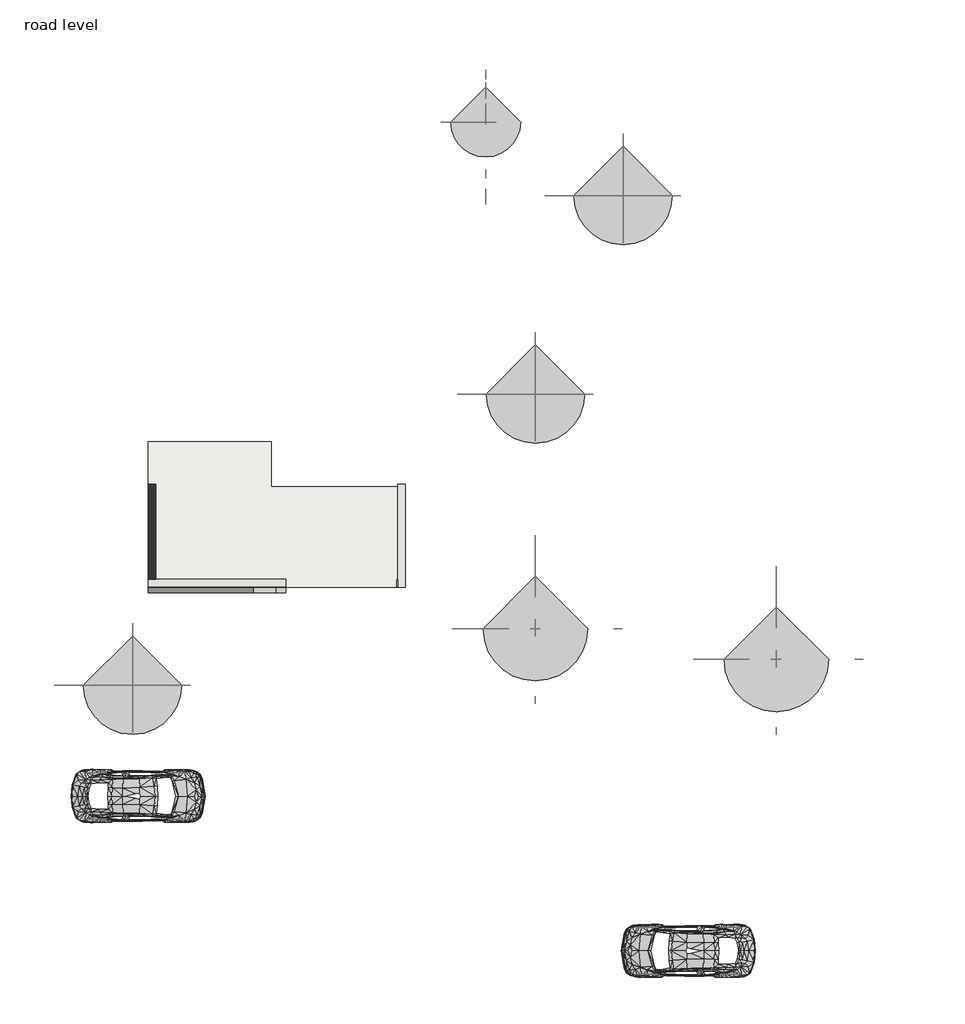
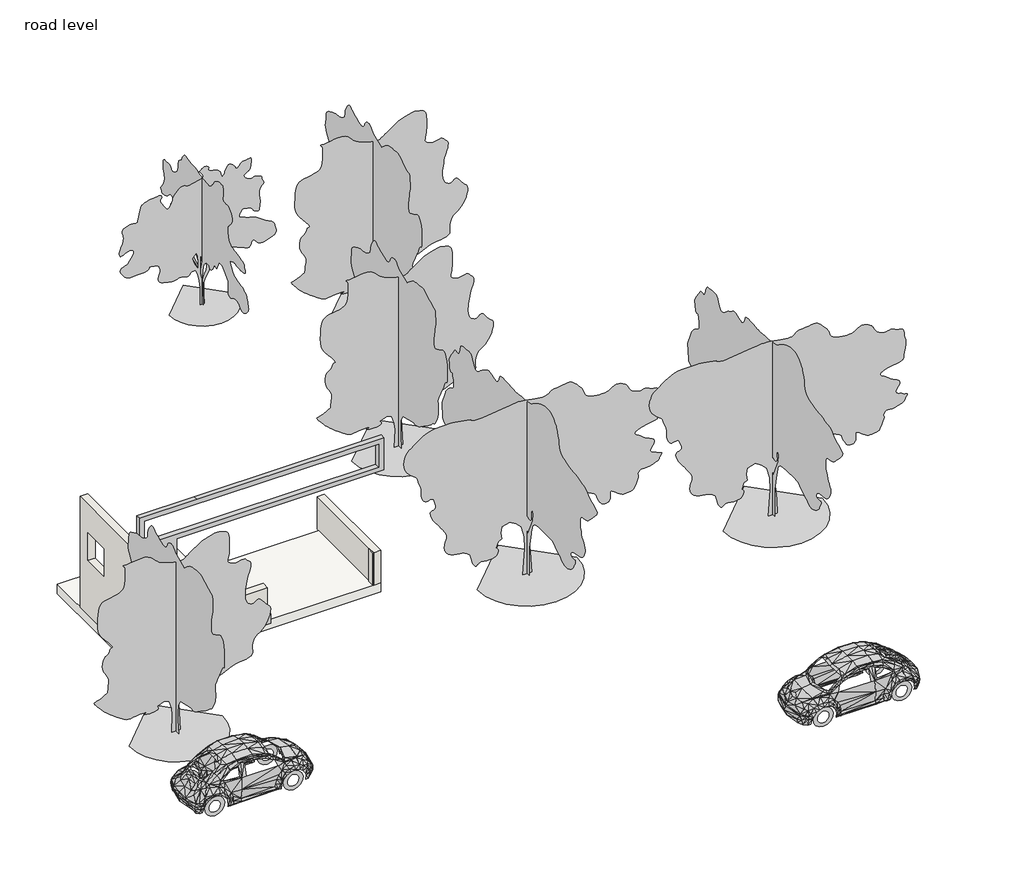
# One storey, incomplete: 6 geographic elements, 4 walls, 2 proxies, 1 furniture element, 1 slab.
"""IFC4 building model written with IfcOpenShell, lengths in millimetres."""

from ifc_helpers import new_model, si_unit, frame, origin, origin_with_axes, place, context, project, spatial, polyline, outline, extrude, faceted_brep, transform, mapped, element, save
from components import rpc_beetle_rpc_beetle_31f8b51e, casework_1_casework_1_0d475414, rpc_tree_deciduous_american_beech_20_b3c041c8, rpc_tree_deciduous_blue_berry_elder_15_a2d70376, rpc_tree_deciduous_common_apple_20_2cf08d23

model = new_model("IFC4")

# Units and contexts
model_context = context("Model", 3, world=origin())
ifc_project = project(units=[si_unit("LENGTHUNIT", "METRE", prefix="MILLI")], contexts=[model_context])

# Site, building, storey
site = spatial("IfcSite", under=ifc_project)
building = spatial("IfcBuilding", under=site)
storey = spatial("IfcBuildingStorey", under=building, Name="road level", Elevation=0.0)

# Proxies
placement = place(None, origin())
rpc_beetle_rpc_beetle_shape = rpc_beetle_rpc_beetle_31f8b51e(model_context)
element("IfcBuildingElementProxy", 1, Name="RPC Beetle : RPC Beetle", ObjectType="RPC Beetle : RPC Beetle", at=placement, inside=storey, context=model_context, shape_type="MappedRepresentation", body=[
    mapped(rpc_beetle_rpc_beetle_shape, transform((36221.8136801, -7466.6247213, -304.8), x_axis=(0.0, 1.0, 0.0), y_axis=(-1.0, 0.0, 0.0), z_axis=(0.0, 0.0, 1.0))),
])
element("IfcBuildingElementProxy", 2, Name="RPC Beetle : RPC Beetle", ObjectType="RPC Beetle : RPC Beetle", at=placement, inside=storey, context=model_context, shape_type="MappedRepresentation", body=[
    mapped(rpc_beetle_rpc_beetle_shape, transform((17489.3136801, -2887.1590687, -304.8), x_axis=(0.0, -1.0, 0.0), y_axis=(1.0, 0.0, 0.0), z_axis=(0.0, 0.0, 1.0))),
])

# Furniture
casework_1_casework_1_shape = casework_1_casework_1_0d475414(model_context)
element("IfcFurniture", 3, ObjectType="Casework 1 : Casework 1", at=placement, inside=storey, context=model_context, shape_type="MappedRepresentation", body=[
    mapped(casework_1_casework_1_shape, transform((0.0, 0.0, 0.0), x_axis=(1.0, 0.0, 0.0), y_axis=(0.0, 1.0, 0.0), z_axis=(0.0, 0.0, 1.0))),
])

# Geographic elements
rpc_tree_deciduous_american_beech_20_shape = rpc_tree_deciduous_american_beech_20_b3c041c8(model_context)
element("IfcGeographicElement", 4, ObjectType="RPC Tree - Deciduous : American Beech - 20'", at=placement, inside=storey, context=model_context, shape_type="MappedRepresentation", body=[
    mapped(rpc_tree_deciduous_american_beech_20_shape, transform((30470.0886189, 9000.0409313, -304.8), x_axis=(1.0, 0.0, 0.0), y_axis=(0.0, 1.0, 0.0), z_axis=(0.0, 0.0, 1.0))),
])
element("IfcGeographicElement", 5, ObjectType="RPC Tree - Deciduous : American Beech - 20'", at=placement, inside=storey, context=model_context, shape_type="MappedRepresentation", body=[
    mapped(rpc_tree_deciduous_american_beech_20_shape, transform((33060.8886189, 14867.4409313, -304.8), x_axis=(1.0, 0.0, 0.0), y_axis=(0.0, 1.0, 0.0), z_axis=(0.0, 0.0, 1.0))),
])
element("IfcGeographicElement", 6, ObjectType="RPC Tree - Deciduous : American Beech - 20'", at=placement, inside=storey, context=model_context, shape_type="MappedRepresentation", body=[
    mapped(rpc_tree_deciduous_american_beech_20_shape, transform((18556.1136801, 389.4409313, -304.8), x_axis=(1.0, 0.0, 0.0), y_axis=(0.0, 1.0, 0.0), z_axis=(0.0, 0.0, 1.0))),
])
rpc_tree_deciduous_blue_berry_elder_15_shape = rpc_tree_deciduous_blue_berry_elder_15_a2d70376(model_context)
element("IfcGeographicElement", 7, ObjectType="RPC Tree - Deciduous : Blue Berry Elder - 15'", at=placement, inside=storey, context=model_context, shape_type="MappedRepresentation", body=[
    mapped(rpc_tree_deciduous_blue_berry_elder_15_shape, transform((28995.5136801, 17044.3752787, 0.0), x_axis=(1.0, 0.0, 0.0), y_axis=(0.0, 1.0, 0.0), z_axis=(0.0, 0.0, 1.0))),
])
rpc_tree_deciduous_common_apple_20_shape = rpc_tree_deciduous_common_apple_20_2cf08d23(model_context)
element("IfcGeographicElement", 8, ObjectType="RPC Tree - Deciduous : Common Apple - 20'", at=placement, inside=storey, context=model_context, shape_type="MappedRepresentation", body=[
    mapped(rpc_tree_deciduous_common_apple_20_shape, transform((37593.4136801, 1151.4409313, -304.8), x_axis=(1.0, 0.0, 0.0), y_axis=(0.0, 1.0, 0.0), z_axis=(0.0, 0.0, 1.0))),
])
element("IfcGeographicElement", 9, ObjectType="RPC Tree - Deciduous : Common Apple - 20'", at=placement, inside=storey, context=model_context, shape_type="MappedRepresentation", body=[
    mapped(rpc_tree_deciduous_common_apple_20_shape, transform((30470.0886189, 2065.8409313, -304.8), x_axis=(1.0, 0.0, 0.0), y_axis=(0.0, 1.0, 0.0), z_axis=(0.0, 0.0, 1.0))),
])

# Slab
element("IfcSlab", 10, ObjectType="Generic - 12\"", at=placement, inside=storey, context=model_context, shape_type="SweptSolid", body=[
    extrude(outline(polyline([(19025.4925873, 7585.6570707), (22657.6925873, 7585.6570707), (22657.6925873, 6256.0880342), (26620.0925873, 6256.0880342), (26620.0925873, 3293.0570707), (19025.4925873, 3293.0570707), (19025.4925873, 7585.6570707)])), frame((0.0, 0.0, -304.8), z_axis=(0.0, 0.0, 1.0), x_axis=(1.0, 0.0, 0.0)), (0.0, 0.0, 1.0), 304.8),
])

# Walls
element("IfcWall", 11, at=placement, inside=storey, context=model_context, shape_type="SweptSolid", body=[
    extrude(outline(polyline([(26366.6136801, 3513.6409313), (26392.0136801, 3513.6409313), (26392.0136801, 3285.0409313), (26366.6136801, 3285.0409313), (26366.6136801, 3513.6409313)])), origin_with_axes(), (0.0, 0.0, 1.0), 1066.8),
])
element("IfcWall", 12, at=placement, inside=storey, context=model_context, shape_type="Brep", body=[
    faceted_brep([(19241.9136801, 3523.1659313, 0.0), (19241.9136801, 6333.0409313, 0.0), (19241.9136801, 6333.0409313, 3657.6), (19241.9136801, 4369.7752787, 3657.6), (19241.9136801, 3523.1659313, 3657.6), (19241.9136801, 5926.6409313, 2708.275), (19241.9136801, 5926.6409313, 1793.875), (19241.9136801, 5063.0409313, 1793.875), (19241.9136801, 5063.0409313, 2708.275), (19013.3136801, 3523.1659313, 0.0), (19013.3136801, 3523.1659313, 1066.8), (19013.3136801, 3523.1659313, 3657.6), (19013.3136801, 6333.0409313, 3657.6), (19013.3136801, 6333.0409313, 609.6), (19013.3136801, 6333.0409313, 0.0), (19013.3136801, 5926.6409313, 2708.275), (19013.3136801, 5063.0409313, 2708.275), (19013.3136801, 5063.0409313, 1793.875), (19013.3136801, 5926.6409313, 1793.875)], [[[0, 1, 2, 3, 4], [5, 6, 7, 8]], [[9, 10, 11, 12, 13, 14], [15, 16, 17, 18]], [[1, 0, 9, 14]], [[0, 4, 11, 10, 9]], [[2, 1, 14, 13, 12]], [[4, 3, 2, 12, 11]], [[6, 5, 15, 18]], [[7, 6, 18, 17]], [[8, 7, 17, 16]], [[5, 8, 16, 15]]]),
])
element("IfcWall", 13, at=placement, inside=storey, context=model_context, shape_type="Brep", body=[
    faceted_brep([(26392.0136801, 6333.0409313, 0.0), (26392.0136801, 3513.6409313, 0.0), (26392.0136801, 3285.0409313, 0.0), (26392.0136801, 3285.0409313, 1066.8), (26392.0136801, 3513.6409313, 1066.8), (26392.0136801, 6333.0409313, 1066.8), (26392.0136801, 6333.0409313, 609.6), (26620.6136801, 6333.0409313, 0.0), (26620.6136801, 6333.0409313, 609.6), (26620.6136801, 6333.0409313, 1066.8), (26620.6136801, 3285.0409313, 1066.8), (26620.6136801, 3285.0409313, 0.0)], [[[0, 1, 2, 3, 4, 5, 6]], [[7, 8, 9, 10, 11]], [[2, 1, 0, 7, 11]], [[5, 4, 3, 10, 9]], [[3, 2, 11, 10]], [[0, 6, 5, 9, 8, 7]]]),
])
element("IfcWall", 14, at=placement, inside=storey, context=model_context, shape_type="Brep", body=[
    faceted_brep([(23090.0136801, 3523.1659313, 0.0), (19241.9136801, 3523.1659313, 0.0), (19013.3136801, 3523.1659313, 0.0), (19013.3136801, 3523.1659313, 1066.8), (23090.0136801, 3523.1659313, 1066.8), (23090.0136801, 3294.5659313, 0.0), (23090.0136801, 3294.5659313, 1066.8), (19013.3136801, 3294.5659313, 1066.8), (19013.3136801, 3294.5659313, 0.0)], [[[0, 1, 2, 3, 4]], [[5, 6, 7, 8]], [[2, 1, 0, 5, 8]], [[4, 3, 7, 6]], [[0, 4, 6, 5]], [[3, 2, 8, 7]]]),
])

save(model, "model.ifc")

# Revit data of these elements
# Type "RPC Beetle : RPC Beetle"
#   built-in parameter 1005198 = "{2, 15},{39, RPC-16-0U6E-L4EG-ENH1-J3KF-SVEL-0TX4-C0},{1, 0},{1, 0},{2, 36},{1, 8},{5, Color},{1, 0},{1, 0},{3, 0.8},{3, 0.8},{3, 0.8},{1, 8},{7, BBoxMin},{1, 0},{1, 0},{1, 0},{1, 0},{1, 0},{1, 8},{7, BBoxMax},{1, 0},{1, 0},{1, 0},{1, 0},{1, 0},{2, 11},{9, RPCTypeId},{1, 0},{1, 0},{39, RPC-16-0U6E-L4EG-ENH1-J3KF-SVEL-0TX4-C0},{1, 6},{14, RPCPlantHeight},{1, 0},{1, 0},{7, 4.91667},{2, 11},{20, AdvancedUIDefinition},{1, 0},{1, 0},{0, },{2, 11},{10, AssetLibID},{1, 0},{1, 0},{36, 4D3F6E72-3F99-4203-98E9-AF80B3C7A7A4},{2, 11},{10, BaseSchema},{1, 0},{1, 0},{9, RPCSchema},{2, 11},{12, ExchangeGUID},{1, 0},{1, 0},{0, },{1, 2},{6, Hidden},{1, 0},{1, 0},{1, 0},{2, 11},{12, LocalizedUID},{1, 0},{1, 0},{0, },{1, 4},{11, RPCCategory},{1, 0},{1, 0},{1, 0},{2, 11},{8, RPCImage},{1, 0},{1, 0},{0, },{1, 4},{13, SchemaVersion},{1, 0},{1, 0},{1, 4},{2, 11},{12, UIDefinition},{1, 0},{1, 0},{0, },{2, 11},{6, UIName},{1, 0},{1, 0},{39, RPC-16-0U6E-L4EG-ENH1-J3KF-SVEL-0TX4-C0},{2, 11},{11, VersionGUID},{1, 0},{1, 0},{9, RPCSchema},{2, 11},{9, assettype},{1, 0},{1, 0},{11, RPCGeometry},{2, 11},{11, description},{1, 0},{1, 0},{0, },{2, 11},{9, localname},{1, 0},{1, 0},{3, RPC},{2, 11},{9, localtype},{1, 0},{1, 0},{3, RPC},{1, 4},{8, revision},{1, 0},{1, 0},{1, 1},{2, 11},{9, thumbnail},{1, 0},{1, 0},{0, },{1, 4},{7, version},{1, 0},{1, 0},{1, 1},{2, 14},{6, Height},{1, 0},{1, 0},{7, 4.91667},{1, 2},{20, RPC_Cast Reflections},{1, 0},{1, 0},{1, 1},{1, 4},{16, RPC_Transparency},{1, 0},{1, 0},{2, 18},{1, 4},{11, RPC_Tinting},{1, 0},{1, 0},{2, 50},{1, 2},{15, RPC_Use Tinting},{1, 0},{1, 0},{1, 0},{1, 2},{17, RPC_License Plate},{1, 0},{1, 0},{1, 0},{2, 11},{25, RPC_License Plate Texture},{1, 0},{1, 0},{64, __RPC:/object data/textures/car/plate/textures/default/rgb/0/0/0},{2, 11},{27, RPC_i_License Plate Texture},{1, 0},{1, 0},{0, },{1, 2},{16, RPC_Custom Plate},{1, 0},{1, 0},{1, 0},{2, 11},{27, RPC_License Plate File Name},{1, 0},{1, 0},{0, },{2, 11},{7, keyword},{1, 0},{1, 0},{27, :Geometry:RPC:VW Beetle [4]},{2, 11},{8, category},{1, 0},{1, 0},{21, :Auto_Economy/Midsize},{21, assetlibrary_base.fbx},{1, 5},"
#   built-in parameter 1005195 = "RPC-16-0U6E-L4EG-ENH1-J3KF-SVEL-0TX4-C0"
#   Height = 0
# Type "RPC Tree - Deciduous : American Beech - 20'"
#   built-in parameter 1005198 = "{2, 15},{39, RPC-16-G1GQ-43Q0-7NP3-0000-ST1L-LVER-AU},{1, 0},{1, 0},{2, 35},{1, 8},{5, Color},{1, 0},{1, 0},{3, 0.8},{3, 0.8},{3, 0.8},{1, 8},{7, BBoxMin},{1, 0},{1, 0},{1, 0},{1, 0},{1, 0},{1, 8},{7, BBoxMax},{1, 0},{1, 0},{1, 0},{1, 0},{1, 0},{2, 11},{9, RPCTypeId},{1, 0},{1, 0},{39, RPC-16-G1GQ-43Q0-7NP3-0000-ST1L-LVER-AU},{1, 6},{14, RPCPlantHeight},{1, 0},{1, 0},{2, 20},{2, 11},{7, keyword},{1, 0},{1, 0},{126, :Geometry:RPC:American Beech:Fagus grandifolia:The beech genus comprises about 10 species; American beech is native to Canada.},{2, 11},{8, category},{1, 0},{1, 0},{16, :Trees [General]},{2, 11},{12, LocalizedUID},{1, 0},{1, 0},{14, American Beech},{2, 14},{6, Height},{1, 0},{1, 0},{2, 20},{1, 2},{16, Cast Reflections},{1, 0},{1, 0},{1, 0},{1, 2},{12, Cast Shadows},{1, 0},{1, 0},{1, 1},{1, 2},{9, Lock View},{1, 0},{1, 0},{1, 0},{1, 4},{5, ViewC},{1, 0},{1, 0},{1, 0},{2, 11},{20, AdvancedUIDefinition},{1, 0},{1, 0},{0, },{2, 11},{10, AssetLibID},{1, 0},{1, 0},{36, 4D3F6E72-3F99-4203-98E9-AF80B3C7A7A4},{2, 11},{10, BaseSchema},{1, 0},{1, 0},{9, RPCSchema},{2, 11},{12, ExchangeGUID},{1, 0},{1, 0},{0, },{1, 2},{6, Hidden},{1, 0},{1, 0},{1, 0},{1, 4},{11, RPCCategory},{1, 0},{1, 0},{1, 0},{2, 11},{8, RPCImage},{1, 0},{1, 0},{0, },{1, 4},{13, SchemaVersion},{1, 0},{1, 0},{1, 4},{2, 11},{12, UIDefinition},{1, 0},{1, 0},{0, },{2, 11},{6, UIName},{1, 0},{1, 0},{39, RPC-16-G1GQ-43Q0-7NP3-0000-ST1L-LVER-AU},{2, 11},{11, VersionGUID},{1, 0},{1, 0},{9, RPCSchema},{2, 11},{9, assettype},{1, 0},{1, 0},{11, RPCGeometry},{2, 11},{11, description},{1, 0},{1, 0},{0, },{2, 11},{9, localname},{1, 0},{1, 0},{3, RPC},{2, 11},{9, localtype},{1, 0},{1, 0},{3, RPC},{1, 4},{8, revision},{1, 0},{1, 0},{1, 1},{2, 11},{9, thumbnail},{1, 0},{1, 0},{0, },{1, 4},{7, version},{1, 0},{1, 0},{1, 1},{1, 2},{20, RPC_Cast Reflections},{1, 0},{1, 0},{1, 1},{1, 2},{16, RPC_Cast Shadows},{1, 0},{1, 0},{1, 1},{1, 2},{13, RPC_Lock View},{1, 0},{1, 0},{1, 0},{1, 4},{9, RPC_ViewC},{1, 0},{1, 0},{1, 0},{21, assetlibrary_base.fbx},{1, 5},"
#   built-in parameter 1005195 = "RPC-16-G1GQ-43Q0-7NP3-0000-ST1L-LVER-AU"
#   Type Comments = "American Beech"
#   Assembly Code = "G2050500"
#   Height = 20' - 0"
#   Default Elevation = 0
# Type "RPC Tree - Deciduous : Blue Berry Elder - 15'"
#   built-in parameter 1005198 = "{2, 15},{39, RPC-16-FWVX-4SXX-5R2N-A000-ST1L-LVER-AU},{1, 0},{1, 0},{2, 35},{1, 8},{5, Color},{1, 0},{1, 0},{3, 0.8},{3, 0.8},{3, 0.8},{1, 8},{7, BBoxMin},{1, 0},{1, 0},{1, 0},{1, 0},{1, 0},{1, 8},{7, BBoxMax},{1, 0},{1, 0},{1, 0},{1, 0},{1, 0},{2, 11},{9, RPCTypeId},{1, 0},{1, 0},{39, RPC-16-FWVX-4SXX-5R2N-A000-ST1L-LVER-AU},{1, 6},{14, RPCPlantHeight},{1, 0},{1, 0},{2, 15},{2, 11},{7, keyword},{1, 0},{1, 0},{285, :Geometry:RPC:Blue-Berry Elder:Sambucus cerulea:Tall:irregularly shaped shrubs or very small trees:up to 10 m high and 20 cm in diameter.  The larger of the Canadian elders; occurs in southern British Columbia in forest clearings:usually on dry open sites with gravelly or stony soils.},{2, 11},{8, category},{1, 0},{1, 0},{16, :Trees [General]},{2, 11},{12, LocalizedUID},{1, 0},{1, 0},{16, Blue-Berry Elder},{2, 14},{6, Height},{1, 0},{1, 0},{2, 15},{1, 2},{16, Cast Reflections},{1, 0},{1, 0},{1, 0},{1, 2},{12, Cast Shadows},{1, 0},{1, 0},{1, 1},{1, 2},{9, Lock View},{1, 0},{1, 0},{1, 0},{1, 4},{5, ViewC},{1, 0},{1, 0},{1, 0},{2, 11},{20, AdvancedUIDefinition},{1, 0},{1, 0},{0, },{2, 11},{10, AssetLibID},{1, 0},{1, 0},{36, 4D3F6E72-3F99-4203-98E9-AF80B3C7A7A4},{2, 11},{10, BaseSchema},{1, 0},{1, 0},{9, RPCSchema},{2, 11},{12, ExchangeGUID},{1, 0},{1, 0},{0, },{1, 2},{6, Hidden},{1, 0},{1, 0},{1, 0},{1, 4},{11, RPCCategory},{1, 0},{1, 0},{1, 0},{2, 11},{8, RPCImage},{1, 0},{1, 0},{0, },{1, 4},{13, SchemaVersion},{1, 0},{1, 0},{1, 4},{2, 11},{12, UIDefinition},{1, 0},{1, 0},{0, },{2, 11},{6, UIName},{1, 0},{1, 0},{39, RPC-16-FWVX-4SXX-5R2N-A000-ST1L-LVER-AU},{2, 11},{11, VersionGUID},{1, 0},{1, 0},{9, RPCSchema},{2, 11},{9, assettype},{1, 0},{1, 0},{11, RPCGeometry},{2, 11},{11, description},{1, 0},{1, 0},{0, },{2, 11},{9, localname},{1, 0},{1, 0},{3, RPC},{2, 11},{9, localtype},{1, 0},{1, 0},{3, RPC},{1, 4},{8, revision},{1, 0},{1, 0},{1, 1},{2, 11},{9, thumbnail},{1, 0},{1, 0},{0, },{1, 4},{7, version},{1, 0},{1, 0},{1, 1},{1, 2},{20, RPC_Cast Reflections},{1, 0},{1, 0},{1, 1},{1, 2},{16, RPC_Cast Shadows},{1, 0},{1, 0},{1, 1},{1, 2},{13, RPC_Lock View},{1, 0},{1, 0},{1, 0},{1, 4},{9, RPC_ViewC},{1, 0},{1, 0},{1, 0},{21, assetlibrary_base.fbx},{1, 5},"
#   built-in parameter 1005195 = "RPC-16-FWVX-4SXX-5R2N-A000-ST1L-LVER-AU"
#   Type Comments = "Blue Berry Elder"
#   Assembly Code = "G2050500"
#   Height = 15' - 0"
#   Default Elevation = 0
# Type "RPC Tree - Deciduous : Common Apple - 20'"
#   built-in parameter 1005198 = "{2, 15},{39, RPC-16-FXGK-4KXX-PJE5-6000-ST1L-LVER-AU},{1, 0},{1, 0},{2, 35},{1, 8},{5, Color},{1, 0},{1, 0},{3, 0.8},{3, 0.8},{3, 0.8},{1, 8},{7, BBoxMin},{1, 0},{1, 0},{1, 0},{1, 0},{1, 0},{1, 8},{7, BBoxMax},{1, 0},{1, 0},{1, 0},{1, 0},{1, 0},{2, 11},{9, RPCTypeId},{1, 0},{1, 0},{39, RPC-16-FXGK-4KXX-PJE5-6000-ST1L-LVER-AU},{1, 6},{14, RPCPlantHeight},{1, 0},{1, 0},{2, 20},{2, 11},{7, keyword},{1, 0},{1, 0},{168, :Geometry:RPC:Common Apple:Malus sylvestris:occurs in southern Ontario near Lakes Erie and Ontario.  Numerous cultivars planted in orchards; naturalized in many places.},{2, 11},{8, category},{1, 0},{1, 0},{16, :Trees [General]},{2, 11},{12, LocalizedUID},{1, 0},{1, 0},{12, Common Apple},{2, 14},{6, Height},{1, 0},{1, 0},{2, 20},{1, 2},{16, Cast Reflections},{1, 0},{1, 0},{1, 0},{1, 2},{12, Cast Shadows},{1, 0},{1, 0},{1, 1},{1, 2},{9, Lock View},{1, 0},{1, 0},{1, 0},{1, 4},{5, ViewC},{1, 0},{1, 0},{1, 0},{2, 11},{20, AdvancedUIDefinition},{1, 0},{1, 0},{0, },{2, 11},{10, AssetLibID},{1, 0},{1, 0},{36, 4D3F6E72-3F99-4203-98E9-AF80B3C7A7A4},{2, 11},{10, BaseSchema},{1, 0},{1, 0},{9, RPCSchema},{2, 11},{12, ExchangeGUID},{1, 0},{1, 0},{0, },{1, 2},{6, Hidden},{1, 0},{1, 0},{1, 0},{1, 4},{11, RPCCategory},{1, 0},{1, 0},{1, 0},{2, 11},{8, RPCImage},{1, 0},{1, 0},{0, },{1, 4},{13, SchemaVersion},{1, 0},{1, 0},{1, 4},{2, 11},{12, UIDefinition},{1, 0},{1, 0},{0, },{2, 11},{6, UIName},{1, 0},{1, 0},{39, RPC-16-FXGK-4KXX-PJE5-6000-ST1L-LVER-AU},{2, 11},{11, VersionGUID},{1, 0},{1, 0},{9, RPCSchema},{2, 11},{9, assettype},{1, 0},{1, 0},{11, RPCGeometry},{2, 11},{11, description},{1, 0},{1, 0},{0, },{2, 11},{9, localname},{1, 0},{1, 0},{3, RPC},{2, 11},{9, localtype},{1, 0},{1, 0},{3, RPC},{1, 4},{8, revision},{1, 0},{1, 0},{1, 1},{2, 11},{9, thumbnail},{1, 0},{1, 0},{0, },{1, 4},{7, version},{1, 0},{1, 0},{1, 1},{1, 2},{20, RPC_Cast Reflections},{1, 0},{1, 0},{1, 1},{1, 2},{16, RPC_Cast Shadows},{1, 0},{1, 0},{1, 1},{1, 2},{13, RPC_Lock View},{1, 0},{1, 0},{1, 0},{1, 4},{9, RPC_ViewC},{1, 0},{1, 0},{1, 0},{21, assetlibrary_base.fbx},{1, 5},"
#   built-in parameter 1005195 = "RPC-16-FXGK-4KXX-PJE5-6000-ST1L-LVER-AU"
#   Type Comments = "Common Apple"
#   Assembly Code = "G2050500"
#   Height = 20' - 0"
#   Default Elevation = 0
# Type "Generic - 12\""
#   Assembly Code = "B1010"
#   Function = 0
#   Layers, outside or top first: 1' - 0" no material (function 1)
# Type
#   Assembly Code = "B2010"
#   Layers, outside or top first: 0' - 9" no material (function 1)
# Elements 1, 2 (IfcBuildingElementProxy, "RPC Beetle : RPC Beetle")
#   Phase Created = New Construction
# Element 3 (IfcFurniture, "Casework 1 : Casework 1")
#   Phase Created = New Construction
#   Materials on its faces: "Birch"
# Elements 4, 5, 6 (IfcGeographicElement, "RPC Tree - Deciduous : American Beech - 20'")
#   Phase Created = New Construction
# Element 7 (IfcGeographicElement, "RPC Tree - Deciduous : Blue Berry Elder - 15'")
#   Phase Created = New Construction
# Elements 8, 9 (IfcGeographicElement, "RPC Tree - Deciduous : Common Apple - 20'")
#   Phase Created = New Construction
# Element 10 (IfcSlab, "Generic - 12\"")
#   Height Offset From Level = 0' - 0"
#   Phase Created = New Construction
#   Materials on its faces: "Default Floor", "Laminate, Ivory, Matte", "Acoustic Ceiling Tile 24 x 24"
# Element 11 (IfcWall)
#   Top Offset = 0' - 0"
#   Base Offset = 0' - 0"
#   Unconnected Height = 3' - 6"
#   wall height = 3' - 6"
#   Phase Created = New Construction
#   Base Constraint = road level
#   Materials on its faces: "Default Wall"
# Element 12 (IfcWall)
#   Top Offset = 0' - 0"
#   Base Offset = 0' - 0"
#   wall height = 12' - 0"
#   Phase Created = New Construction
#   Base Constraint = road level
#   Top Constraint = 1st floor
#   Materials on its faces: "Default Wall", "Laminate, Ivory, Matte"
# Elements 13, 14 (IfcWall)
#   Top Offset = 0' - 0"
#   Base Offset = 0' - 0"
#   Unconnected Height = 3' - 6"
#   wall height = 3' - 6"
#   Phase Created = New Construction
#   Base Constraint = road level
#   Materials on its faces: "Laminate, Ivory, Matte", "Default Wall", "Birch"
# Materials
#   "Birch": class "Wood", colour RGB 224 178 126, transparency 0, Description = "Betula Alleghaniensis", Cost = 0
#   "Default Floor": colour RGB 128 128 128, transparency 0, Cost = 0
#   "Laminate, Ivory, Matte": class "Plastic", colour RGB 247 247 239, transparency 0, Description = "Plastic Laminate - Ivory, Matte", Cost = 0
#   "Acoustic Ceiling Tile 24 x 24": class "Generic", colour RGB 232 232 232, transparency 0, Description = "Acoustic Ceiling Tile 24 x 24", Cost = 0
#   "Default Wall": colour RGB 128 128 128, transparency 0, Cost = 0
